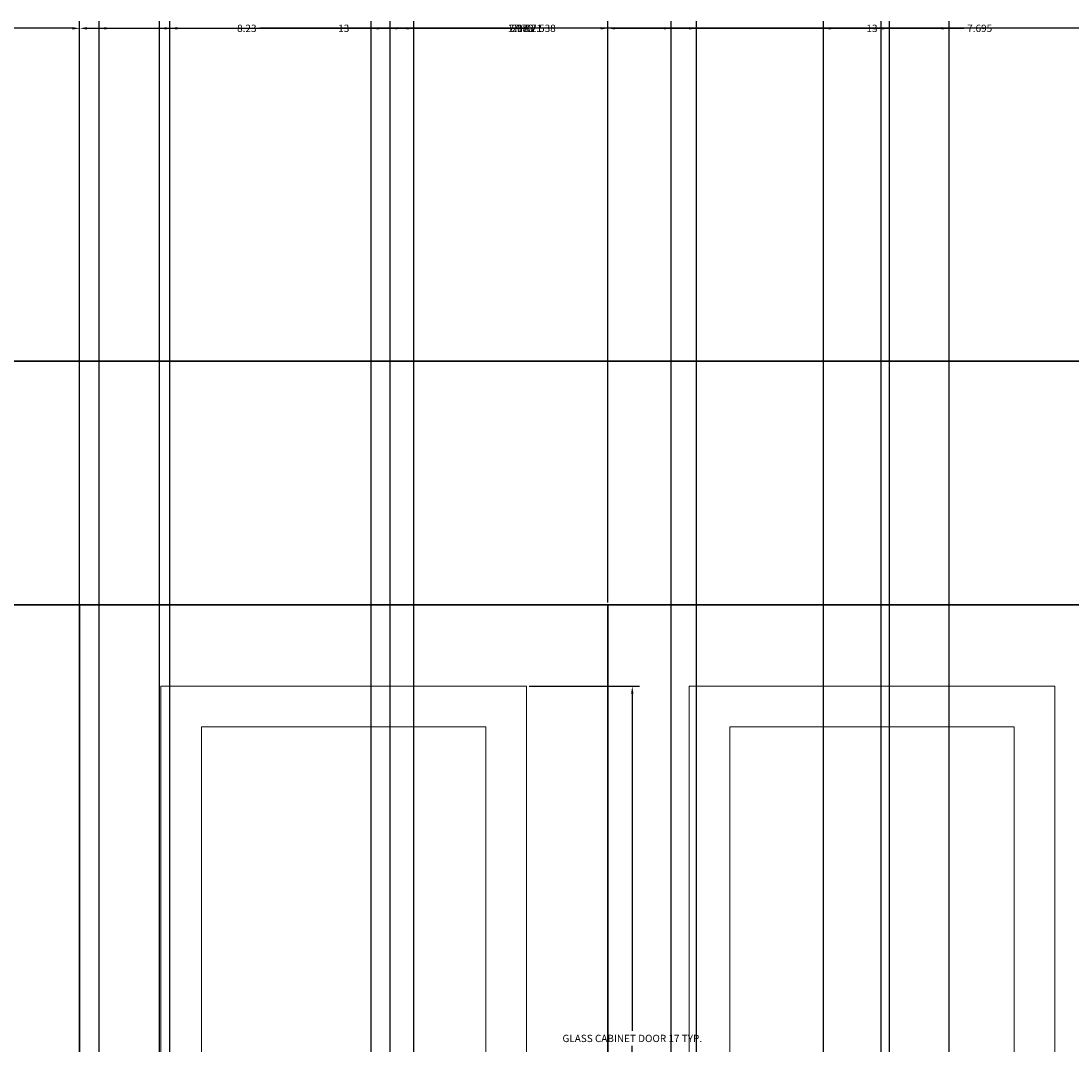
# Model space of a CAD drawing. Units: inches. Extents: x 27 to 200, y -50 to 102.
# Tile 20 of 26: x 119 to 145, y 77 to 102. Entities that reach past the tile are written whole.
import ezdxf

# ---------------------------------------------------------------- set-up
doc = ezdxf.new("R2010")
doc.units = ezdxf.units.IN
doc.header["$MEASUREMENT"] = 0
for name, color, linetype, lineweight in [('A-ANNO-DIMS', 2, 'Continuous', 18), ('A-ELEV', 7, 'Continuous', 35), ('A-FURN', 8, 'Continuous', 18)]:
    doc.layers.add(name, color=color, linetype=linetype, lineweight=lineweight)
doc.styles.get("Standard").update_dxf_attribs({"font": 'arial.ttf'})
doc.dimstyles.get("Standard").update_dxf_attribs({"dimtxt": 0.18, "dimasz": 0.18, "dimexe": 0.18, "dimexo": 0.0625, "dimgap": 0.09, "dimtad": 0, "dimtih": 1, "dimtoh": 1, "dimdec": 4, "dimzin": 0, "dimdsep": 46, "dimtxsty": 'Standard', "dimcen": 0.09, "dimadec": 0, "dimazin": 0, "dimtfac": 1, "dimtdec": 4, "dimtofl": 0, "dimtmove": 0, "dimatfit": 3, "dimfxl": 1, "dimtolj": 1, "dimtzin": 0, "dimarcsym": 0})

# ---------------------------------------------------------------- blocks, each defined once
blk = doc.blocks.new('CAB-DOOR-GLASS')
for p, q in [((0, 17.345), (9, 17.345)), ((0, 0), (0, 17.345)), ((9, 17.345), (9, 0)), ((1, 16.345), (8, 16.345)), ((1, 0), (1, 16.345)), ((8, 16.345), (8, 0)), ((9, 0), (0, 0))]:
    blk.add_line(p, q)
blk = doc.blocks.new('*D9')
at = {"layer": 'A-ANNO-DIMS', "color": 0, "lineweight": -2, "transparency": 16777216}
for p, q in [((131.479, 85.926), (134.199, 85.926)), ((134.019, 85.746), (134.019, 77.437)), ((134.019, 68.761), (134.019, 77.071)), ((131.479, 68.581), (134.199, 68.581))]:
    blk.add_line(p, q, dxfattribs=at)
at = {"layer": 'A-ANNO-DIMS', "color": 0, "transparency": 16777216}
for points in [[(133.989, 85.746), (134.049, 85.746), (134.019, 85.926)], [(133.989, 68.761), (134.049, 68.761), (134.019, 68.581)]]:
    blk.add_solid(points, dxfattribs=at)
at = {"layer": 'Defpoints', "color": 0, "transparency": 16777216}
for p in [(131.417, 85.926), (134.019, 85.926), (131.417, 68.581)]:
    blk.add_point(p, dxfattribs=at)
at = {"layer": 'A-ANNO-DIMS', "color": 0, "transparency": 16777216, "insert": (134.019, 77.254), "char_height": 0.18, "attachment_point": 5}
blk.add_mtext('\\A1;GLASS CABINET DOOR 17 TYP.', dxfattribs=at)
blk = doc.blocks.new('*D17')
at = {"layer": 'A-ANNO-DIMS', "color": 0, "lineweight": -2, "transparency": 16777216}
for p, q in [((102.417, 87.989), (102.417, 102.306)), ((102.597, 102.126), (111.206, 102.126)), ((120.237, 102.126), (111.628, 102.126)), ((120.417, 87.989), (120.417, 102.306))]:
    blk.add_line(p, q, dxfattribs=at)
at = {"layer": 'A-ANNO-DIMS', "color": 0, "transparency": 16777216}
for points in [[(102.597, 102.156), (102.597, 102.096), (102.417, 102.126)], [(120.237, 102.156), (120.237, 102.096), (120.417, 102.126)]]:
    blk.add_solid(points, dxfattribs=at)
at = {"layer": 'Defpoints', "color": 0, "transparency": 16777216}
for p in [(120.417, 102.126), (102.417, 87.926), (120.417, 87.926)]:
    blk.add_point(p, dxfattribs=at)
at = {"layer": 'A-ANNO-DIMS', "color": 0, "transparency": 16777216, "insert": (111.417, 102.126), "char_height": 0.18, "attachment_point": 5}
blk.add_mtext('\\A1;18', dxfattribs=at)
blk = doc.blocks.new('*D18')
at = {"layer": 'A-ANNO-DIMS', "color": 0, "lineweight": -2, "transparency": 16777216}
for p, q in [((120.417, 87.989), (120.417, 102.306)), ((120.597, 102.126), (126.706, 102.126)), ((133.237, 102.126), (127.127, 102.126)), ((133.417, 87.989), (133.417, 102.306))]:
    blk.add_line(p, q, dxfattribs=at)
at = {"layer": 'A-ANNO-DIMS', "color": 0, "transparency": 16777216}
for points in [[(120.597, 102.156), (120.597, 102.096), (120.417, 102.126)], [(133.237, 102.156), (133.237, 102.096), (133.417, 102.126)]]:
    blk.add_solid(points, dxfattribs=at)
at = {"layer": 'Defpoints', "color": 0, "transparency": 16777216}
for p in [(133.417, 102.126), (120.417, 87.926), (133.417, 87.926)]:
    blk.add_point(p, dxfattribs=at)
at = {"layer": 'A-ANNO-DIMS', "color": 0, "transparency": 16777216, "insert": (126.917, 102.126), "char_height": 0.18, "attachment_point": 5}
blk.add_mtext('\\A1;13', dxfattribs=at)
blk = doc.blocks.new('*D19')
at = {"layer": 'A-ANNO-DIMS', "color": 0, "lineweight": -2, "transparency": 16777216}
for p, q in [((133.417, 87.989), (133.417, 102.306)), ((133.597, 102.126), (139.706, 102.126)), ((146.237, 102.126), (140.127, 102.126)), ((146.417, 87.989), (146.417, 102.306))]:
    blk.add_line(p, q, dxfattribs=at)
at = {"layer": 'A-ANNO-DIMS', "color": 0, "transparency": 16777216}
for points in [[(133.597, 102.156), (133.597, 102.096), (133.417, 102.126)], [(146.237, 102.156), (146.237, 102.096), (146.417, 102.126)]]:
    blk.add_solid(points, dxfattribs=at)
at = {"layer": 'Defpoints', "color": 0, "transparency": 16777216}
for p in [(146.417, 102.126), (133.417, 87.926), (146.417, 87.926)]:
    blk.add_point(p, dxfattribs=at)
at = {"layer": 'A-ANNO-DIMS', "color": 0, "transparency": 16777216, "insert": (139.917, 102.126), "char_height": 0.18, "attachment_point": 5}
blk.add_mtext('\\A1;13', dxfattribs=at)
blk = doc.blocks.new('*D49')
at = {"layer": 'A-ANNO-DIMS', "color": 0, "lineweight": -2, "transparency": 16777216}
for p, q in [((120.417, 51.989), (120.417, 102.306)), ((120.597, 102.126), (124.208, 102.126)), ((128.466, 102.126), (124.856, 102.126)), ((128.646, 51.989), (128.646, 102.306))]:
    blk.add_line(p, q, dxfattribs=at)
at = {"layer": 'A-ANNO-DIMS', "color": 0, "transparency": 16777216}
for points in [[(120.597, 102.156), (120.597, 102.096), (120.417, 102.126)], [(128.466, 102.156), (128.466, 102.096), (128.646, 102.126)]]:
    blk.add_solid(points, dxfattribs=at)
at = {"layer": 'Defpoints', "color": 0, "transparency": 16777216}
for p in [(128.646, 102.126), (120.417, 51.926), (128.646, 51.926)]:
    blk.add_point(p, dxfattribs=at)
at = {"layer": 'A-ANNO-DIMS', "color": 0, "transparency": 16777216, "insert": (124.532, 102.126), "char_height": 0.18, "attachment_point": 5}
blk.add_mtext('\\A1;8.23', dxfattribs=at)
blk = doc.blocks.new('*D50')
at = {"layer": 'A-ANNO-DIMS', "color": 0, "lineweight": -2, "transparency": 16777216}
for p, q in [((138.722, 51.989), (138.722, 102.306)), ((138.902, 102.126), (142.176, 102.126)), ((146.237, 102.126), (142.963, 102.126)), ((146.417, 51.989), (146.417, 102.306))]:
    blk.add_line(p, q, dxfattribs=at)
at = {"layer": 'A-ANNO-DIMS', "color": 0, "transparency": 16777216}
for points in [[(138.902, 102.156), (138.902, 102.096), (138.722, 102.126)], [(146.237, 102.156), (146.237, 102.096), (146.417, 102.126)]]:
    blk.add_solid(points, dxfattribs=at)
at = {"layer": 'Defpoints', "color": 0, "transparency": 16777216}
for p in [(146.417, 102.126), (138.722, 51.926), (146.417, 51.926)]:
    blk.add_point(p, dxfattribs=at)
at = {"layer": 'A-ANNO-DIMS', "color": 0, "transparency": 16777216, "insert": (142.569, 102.126), "char_height": 0.18, "attachment_point": 5}
blk.add_mtext('\\A1;7.695', dxfattribs=at)
blk = doc.blocks.new('*D53')
at = {"layer": 'A-ANNO-DIMS', "color": 0, "lineweight": -2, "transparency": 16777216}
for p, q in [((120.895, 14.04), (120.895, 102.306)), ((121.075, 102.126), (130.962, 102.126)), ((141.636, 102.126), (131.75, 102.126)), ((141.816, 14.04), (141.816, 102.306))]:
    blk.add_line(p, q, dxfattribs=at)
at = {"layer": 'A-ANNO-DIMS', "color": 0, "transparency": 16777216}
for points in [[(121.075, 102.156), (121.075, 102.096), (120.895, 102.126)], [(141.636, 102.156), (141.636, 102.096), (141.816, 102.126)]]:
    blk.add_solid(points, dxfattribs=at)
at = {"layer": 'Defpoints', "color": 0, "transparency": 16777216}
for p in [(141.816, 102.126), (120.895, 13.977), (141.816, 13.977)]:
    blk.add_point(p, dxfattribs=at)
at = {"layer": 'A-ANNO-DIMS', "color": 0, "transparency": 16777216, "insert": (131.356, 102.126), "char_height": 0.18, "attachment_point": 5}
blk.add_mtext('\\A1;20.92', dxfattribs=at)
blk = doc.blocks.new('*D57')
at = {"layer": 'A-ANNO-DIMS', "color": 0, "lineweight": -2, "transparency": 16777216}
for p, q in [((122.38, 4.48), (122.38, 102.306)), ((122.56, 102.126), (130.875, 102.126)), ((139.961, 102.126), (131.645, 102.126)), ((140.141, 4.48), (140.141, 102.306))]:
    blk.add_line(p, q, dxfattribs=at)
at = {"layer": 'A-ANNO-DIMS', "color": 0, "transparency": 16777216}
for points in [[(122.56, 102.156), (122.56, 102.096), (122.38, 102.126)], [(139.961, 102.156), (139.961, 102.096), (140.141, 102.126)]]:
    blk.add_solid(points, dxfattribs=at)
at = {"layer": 'Defpoints', "color": 0, "transparency": 16777216}
for p in [(140.141, 102.126), (122.38, 4.418), (140.141, 4.418)]:
    blk.add_point(p, dxfattribs=at)
at = {"layer": 'A-ANNO-DIMS', "color": 0, "transparency": 16777216, "insert": (131.26, 102.126), "char_height": 0.18, "attachment_point": 5}
blk.add_mtext('\\A1;17.76', dxfattribs=at)
blk = doc.blocks.new('*D59')
at = {"layer": 'A-ANNO-DIMS', "color": 0, "lineweight": -2, "transparency": 16777216}
for p, q in [((127.595, -0.162), (127.595, 102.306)), ((127.775, 102.126), (130.893, 102.126)), ((134.798, 102.126), (131.679, 102.126)), ((134.978, -0.162), (134.978, 102.306))]:
    blk.add_line(p, q, dxfattribs=at)
at = {"layer": 'A-ANNO-DIMS', "color": 0, "transparency": 16777216}
for points in [[(127.775, 102.156), (127.775, 102.096), (127.595, 102.126)], [(134.798, 102.156), (134.798, 102.096), (134.978, 102.126)]]:
    blk.add_solid(points, dxfattribs=at)
at = {"layer": 'Defpoints', "color": 0, "transparency": 16777216}
for p in [(134.978, 102.126), (127.595, -0.225), (134.978, -0.225)]:
    blk.add_point(p, dxfattribs=at)
at = {"layer": 'A-ANNO-DIMS', "color": 0, "transparency": 16777216, "insert": (131.286, 102.126), "char_height": 0.18, "attachment_point": 5}
blk.add_mtext('\\A1;7.383', dxfattribs=at)
blk = doc.blocks.new('*D61')
at = {"layer": 'A-ANNO-DIMS', "color": 0, "lineweight": -2, "transparency": 16777216}
for p, q in [((122.638, -4.237), (122.638, 102.306)), ((122.818, 102.126), (131.125, 102.126)), ((140.167, 102.126), (131.86, 102.126)), ((140.347, -4.237), (140.347, 102.306))]:
    blk.add_line(p, q, dxfattribs=at)
at = {"layer": 'A-ANNO-DIMS', "color": 0, "transparency": 16777216}
for points in [[(122.818, 102.156), (122.818, 102.096), (122.638, 102.126)], [(140.167, 102.156), (140.167, 102.096), (140.347, 102.126)]]:
    blk.add_solid(points, dxfattribs=at)
at = {"layer": 'Defpoints', "color": 0, "transparency": 16777216}
for p in [(140.347, 102.126), (122.638, -4.3), (140.347, -4.3)]:
    blk.add_point(p, dxfattribs=at)
at = {"layer": 'A-ANNO-DIMS', "color": 0, "transparency": 16777216, "insert": (131.493, 102.126), "char_height": 0.18, "attachment_point": 5}
blk.add_mtext('\\A1;17.71', dxfattribs=at)
blk = doc.blocks.new('*D63')
at = {"layer": 'A-ANNO-DIMS', "color": 0, "lineweight": -2, "transparency": 16777216}
for p, q in [((128.059, -9.034), (128.059, 102.306)), ((128.239, 102.126), (131.435, 102.126)), ((135.417, 102.126), (132.221, 102.126)), ((135.597, -9.034), (135.597, 102.306))]:
    blk.add_line(p, q, dxfattribs=at)
at = {"layer": 'A-ANNO-DIMS', "color": 0, "transparency": 16777216}
for points in [[(128.239, 102.156), (128.239, 102.096), (128.059, 102.126)], [(135.417, 102.156), (135.417, 102.096), (135.597, 102.126)]]:
    blk.add_solid(points, dxfattribs=at)
at = {"layer": 'Defpoints', "color": 0, "transparency": 16777216}
for p in [(135.597, 102.126), (128.059, -9.097), (135.597, -9.097)]:
    blk.add_point(p, dxfattribs=at)
at = {"layer": 'A-ANNO-DIMS', "color": 0, "transparency": 16777216, "insert": (131.828, 102.126), "char_height": 0.18, "attachment_point": 5}
blk.add_mtext('\\A1;7.538', dxfattribs=at)

msp = doc.modelspace()

# ---------------------------------------------------------------- linework, layer by layer
at = {"layer": 'A-ELEV'}
for p, q in [((191.4169, 93.9264), (35.4169, 93.9264)), ((191.4169, 87.9264), (35.4169, 87.9264)), ((120.4169, 87.9264), (120.4169, 51.9264)), ((133.4169, 87.9264), (133.4169, 51.9264))]:
    msp.add_line(p, q, dxfattribs=at)

# ---------------------------------------------------------------- block references
at = {"layer": 'A-FURN'}
for p in [(122.417, 68.581), (135.417, 68.581)]:
    msp.add_blockref('CAB-DOOR-GLASS', p, dxfattribs=at)

# ---------------------------------------------------------------- dimensions: what is measured, and where the dimension line sits
at = {"layer": 'A-ANNO-DIMS'}
for base, p1, p2, override, picture, middle in [((120.4169, 102.1264), (102.4169, 87.9264), (120.4169, 87.9264), {"dimdec": 0, "dimlfac": 1, "dimrnd": 0, "dimzin": 0, "dimdsep": 46, "dimlunit": 2}, '*D17', (111.4169, 102.1264)), ((133.4169, 102.1264), (120.4169, 87.9264), (133.4169, 87.9264), {"dimdec": 0, "dimlfac": 1, "dimrnd": 0, "dimzin": 0, "dimdsep": 46, "dimlunit": 2}, '*D18', (126.9169, 102.1264)), ((128.6463, 102.1264), (120.4169, 51.9264), (128.6463, 51.9264), {"dimdec": 2, "dimlfac": 1, "dimrnd": 0, "dimzin": 0, "dimdsep": 46, "dimlunit": 2}, '*D49', (124.5316, 102.1264)), ((141.8163, 102.1264), (120.8954, 13.9773), (141.8163, 13.9773), {"dimdec": 2, "dimlfac": 1, "dimrnd": 0, "dimzin": 0, "dimdsep": 46, "dimlunit": 2}, '*D53', (131.3558, 102.1264)), ((140.1406, 102.1264), (122.38, 4.4177), (140.1406, 4.4177), {"dimdec": 2, "dimlfac": 1, "dimrnd": 0, "dimzin": 0, "dimdsep": 46, "dimlunit": 2}, '*D57', (131.2603, 102.1264)), ((140.3471, 102.1264), (122.6381, -4.2997), (140.3471, -4.2997), {"dimdec": 2, "dimlfac": 1, "dimrnd": 0, "dimzin": 0, "dimdsep": 46, "dimlunit": 2}, '*D61', (131.4926, 102.1264)), ((134.9776, 102.1264), (127.5946, -0.2247), (134.9776, -0.2247), {"dimdec": 3, "dimlfac": 1, "dimrnd": 0, "dimzin": 0, "dimdsep": 46, "dimlunit": 2}, '*D59', (131.2861, 102.1264)), ((135.5972, 102.1264), (128.0592, -9.0968), (135.5972, -9.0968), {"dimdec": 3, "dimlfac": 1, "dimrnd": 0, "dimzin": 0, "dimdsep": 46, "dimlunit": 2}, '*D63', (131.8282, 102.1264)), ((146.4169, 102.1264), (133.4169, 87.9264), (146.4169, 87.9264), {"dimdec": 0, "dimlfac": 1, "dimrnd": 0, "dimzin": 0, "dimdsep": 46, "dimlunit": 2}, '*D19', (139.9169, 102.1264)), ((146.4169, 102.1264), (138.7218, 51.9264), (146.4169, 51.9264), {"dimdec": 3, "dimlfac": 1, "dimrnd": 0, "dimzin": 0, "dimdsep": 46, "dimlunit": 2}, '*D50', (142.5694, 102.1264))]:
    dim = msp.add_linear_dim(base=base, p1=p1, p2=p2, dimstyle='Standard', override=override, dxfattribs=at)
    dim.commit()
    dim.dimension.update_dxf_attribs({"geometry": picture, "text_midpoint": middle})
dim = msp.add_linear_dim(base=(134.0187, 85.9264), p1=(131.4169, 68.5812), p2=(131.4169, 85.9264), angle=90, text='GLASS CABINET DOOR <> TYP.', dimstyle='Standard', override={"dimdec": 0, "dimrnd": 0, "dimzin": 0, "dimlunit": 2}, dxfattribs=at)
dim.commit()
dim.dimension.update_dxf_attribs({"geometry": '*D9', "text_midpoint": (134.0187, 77.2538)})

doc.saveas('drawing.dxf')
